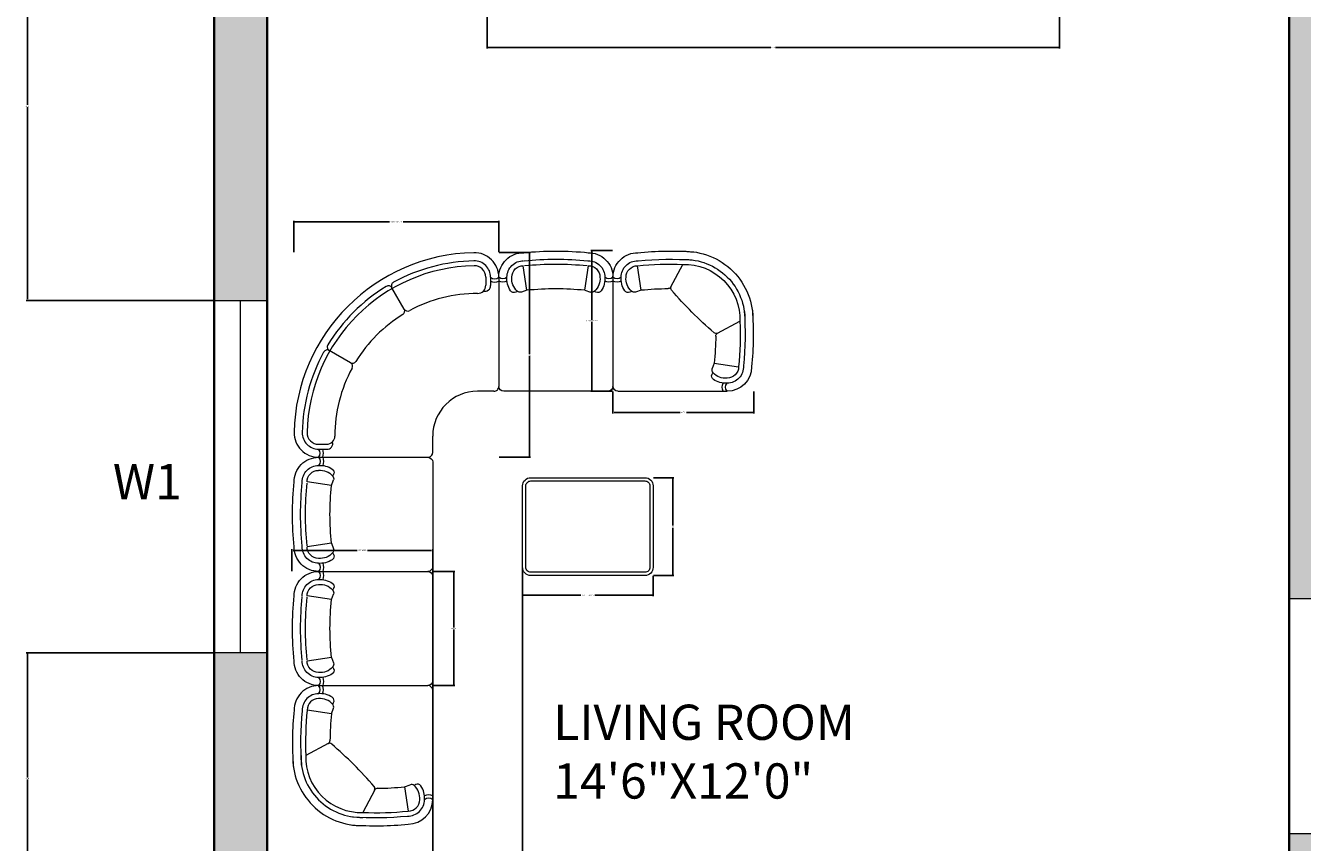
# Model space of a CAD drawing. Units: inches. Extents: x 5 to 421, y -617 to 43.
# Tile 6 of 15: x 5 to 223, y -385 to -246. Entities that reach past the tile are written whole.
import ezdxf

# ---------------------------------------------------------------- set-up
doc = ezdxf.new("R2010")
doc.units = ezdxf.units.IN
doc.header["$MEASUREMENT"] = 0
for name, color, linetype, lineweight in [('A-ANNO-DIMS', 2, 'Continuous', 18), ('A-ANNO-TEXT', 7, 'Continuous', 18), ('A-AREA-IDEN', 7, 'Continuous', 25), ('A-DOOR', 4, 'Continuous', 20), ('A-FURN', 8, 'Continuous', 13), ('A-GLAZ', 4, 'Continuous', 18), ('A-WALL', 7, 'Continuous', 35)]:
    doc.layers.add(name, color=color, linetype=linetype, lineweight=lineweight)
doc.layers.add('A-WALL-PATT', color=251, linetype='Continuous', lineweight=13, true_color=0x636466)
doc.styles.get("Standard").update_dxf_attribs({"font": 'arial.ttf'})
doc.dimstyles.get("Standard").update_dxf_attribs({"dimtxt": 0.18, "dimasz": 0.18, "dimexe": 0.18, "dimexo": 0.0625, "dimgap": 0.09, "dimtad": 0, "dimtih": 1, "dimtoh": 1, "dimdec": 0, "dimzin": 0, "dimdsep": 46, "dimlunit": 3, "dimtxsty": 'Standard', "dimcen": 0.09, "dimadec": 0, "dimazin": 0, "dimtfac": 1, "dimtdec": 0, "dimtofl": 0, "dimtmove": 0, "dimatfit": 3, "dimfxl": 1, "dimtolj": 1, "dimtzin": 0, "dimarcsym": 0})

# ---------------------------------------------------------------- blocks, each defined once
blk = doc.blocks.new('A$C707258B2')
at = {"color": 0}
for p, q in [((0.4042, 0.342), (1.0739, 0.342)), ((0.4042, 0.292), (0.4544, 0.292)), ((0.4042, 0.262), (0.4539, 0.262)), ((1.1039, 0.312), (1.1039, 0.212)), ((1.4789, -0.063), (1.3789, -0.063)), ((1.5089, -0.7628), (1.5089, -0.093)), ((0.5998, -0.2378), (0.4699, -0.3128)), ((0.9291, -0.5671), (0.8541, -0.697)), ((1.4289, -0.7628), (1.4289, -0.713)), ((1.4589, -0.7628), (1.4589, -0.7125))]:
    blk.add_line(p, q, dxfattribs=at)
for centre, radius, start, end in [((0.4042, 0.192), 0.15, 90, 181.17538), ((0.3779, 0.317), 0.0362, 316.39718, 43.60282), ((0.3679, 0.317), 0.0662, 337.82984, 22.17016), ((1.0739, 0.312), 0.03, 360, 90), ((0.4042, 0.192), 0.1, 90, 181.17538), ((0.4042, 0.192), 0.07, 90, 181.17538), ((0.4539, 0.212), 0.05, 360, 90), ((0.4548, 0.2564), 0.0357, 345.42616, 90.55549), ((1.3789, 0.212), 1.125, 181.17538, 268.82462), ((1.3789, 0.212), 1.075, 181.17538, 208.63569), ((1.3789, 0.212), 1.045, 181.17538, 268.82462), ((1.3789, 0.212), 0.875, 180, 208.40825), ((1.3789, 0.212), 0.275, 180, 270), ((1.4789, -0.093), 0.03, 360, 90), ((0.5873, -0.2162), 0.025, 300, 28.40825), ((0.6123, -0.2595), 0.025, 31.59175, 120), ((0.4574, -0.2912), 0.025, 208.63569, 300), ((0.4824, -0.3345), 0.025, 120, 211.36431), ((1.3789, 0.212), 0.875, 211.59175, 238.40825), ((1.3789, 0.212), 1.075, 211.36431, 238.63569), ((0.9075, -0.5546), 0.025, 330, 58.40825), ((0.9508, -0.5796), 0.025, 61.59175, 150), ((1.3789, 0.212), 0.875, 241.59175, 270), ((0.8324, -0.6845), 0.025, 238.63569, 330), ((0.8757, -0.7095), 0.025, 150, 241.36431), ((1.3789, -0.713), 0.05, 360, 90), ((1.4255, -0.7093), 0.0336, 354.63008, 109.38826), ((1.3789, 0.212), 1.075, 241.36431, 268.82462), ((1.3589, -0.7628), 0.15, 268.82462, 360), ((1.3589, -0.7628), 0.1, 268.82462, 360), ((1.3589, -0.7628), 0.07, 268.82462, 360), ((1.4839, -0.7988), 0.0662, 67.82984, 112.17016), ((1.4839, -0.789), 0.0362, 46.39718, 133.60282)]:
    blk.add_arc(centre, radius, start, end, dxfattribs=at)
blk = doc.blocks.new('A$C1352')
at = {"color": 0}
for points in [[(0.0027, 0.053), (0.0027, 0.553, -0.414214), (0.0527, 0.603), (0.7527, 0.603, -0.414214), (0.8027, 0.553), (0.8027, 0.053, -0.414214), (0.7527, 0.003), (0.0527, 0.003, -0.414214)], [(0.0227, 0.053), (0.0227, 0.553, -0.414214), (0.0527, 0.583), (0.7527, 0.583, -0.414214), (0.7827, 0.553), (0.7827, 0.053, -0.414214), (0.7527, 0.023), (0.0527, 0.023, -0.414214)]]:
    blk.add_lwpolyline(points, format="xyb", close=True, dxfattribs=at)
blk = doc.blocks.new('part 01')
at = {"color": 0}
for p, q in [((-669.8, 700), (0, 700)), ((30, 30), (30, 670)), ((-590.9, 527.1), (-739.8, 550)), ((-590.9, 527.1), (-578.5, 561.2)), ((-590.9, 172.9), (-739.8, 150)), ((-590.9, 172.9), (-578.5, 138.8)), ((-669.8, 0), (0, 0))]:
    blk.add_line(p, q, dxfattribs=at)
for centre, radius, start, end in [((-669.8, 550), 150, 90, 181.17538), ((-669.8, 550), 100, 90, 181.17538), ((-659.7, 517.8), 132.7, 56.08973, 95.61316), ((-696, 675), 36.2, 316.39718, 43.60282), ((-705.9, 675), 66.2, 337.82984, 22.17016), ((-599.7, 607.2), 25, 332.96082, 56.08973), ((0, 670), 30, 0, 90), ((1178.1, 350), 2007.9, 174.28354, 185.71646), ((-669.8, 550), 70, 90, 181.17538), ((-659.7, 517.8), 102.7, 42.00663, 95.61316), ((-624.8, 620), 53.2, 321.00172, 332.96082), ((-602, 569.8), 25, 340, 42.00663), ((1178.1, 350), 1957.9, 174.28354, 185.71646), ((1178.1, 350), 1927.9, 174.28354, 185.71646), ((1178.1, 350), 1777.9, 174.28354, 185.71646), ((-669.8, 150), 150, 178.82462, 270), ((-669.8, 150), 100, 178.82462, 270), ((-669.8, 150), 70, 178.82462, 270), ((-659.7, 182.2), 102.7, 264.38684, 317.99337), ((-599.7, 92.8), 25, 303.91027, 27.03918), ((-602, 130.2), 25, 317.99337, 20), ((-624.8, 80), 53.2, 27.03918, 38.99828), ((-659.7, 182.2), 132.7, 264.38684, 303.91027), ((-696, 25), 36.2, 316.39718, 43.60282), ((-705.9, 25), 66.2, 337.82984, 22.17016), ((0, 30), 30, 270, 0)]:
    blk.add_arc(centre, radius, start, end, dxfattribs=at)
blk = doc.blocks.new('part02')
at = {"color": 0}
for p, q in [((0, -669.8), (0, 0)), ((30, 30), (699.8, 30)), ((620.9, -142.9), (608.5, -108.8)), ((620.9, -142.9), (769.8, -120)), ((640.4, -325.6), (778.2, -398.9)), ((172.9, -590.9), (138.8, -578.5)), ((172.9, -590.9), (150, -739.8)), ((355.6, -610.4), (428.9, -748.2))]:
    blk.add_line(p, q, dxfattribs=at)
for centre, radius, start, end in [((30, 0), 30, 90, 180), ((726, 5), 56.2, 153.6122, 206.66656), ((726, 5), 36.2, 136.39718, 223.60282), ((699.8, -120), 150, 0, 90), ((629.7, -62.8), 25, 123.91027, 207.03918), ((654.8, -50), 53.2, 207.03918, 218.99828), ((689.7, -152.2), 102.7, 84.38684, 137.99337), ((689.3, -151.3), 131.7, 85.43775, 123.98866), ((699.5, -120.6), 100.6, 357.50055, 89.85796), ((699.8, -120), 70, 0, 90), ((632, -100.2), 25, 137.99337, 200), ((-1148.1, -320), 1777.9, 0.38365, 5.71646), ((-1228.2, -319.5), 2007.9, 357.73494, 5.70316), ((-1148.1, -320), 1957.9, 355.86566, 5.71646), ((-1148.1, -320), 2007.9, 355.81801, 5.71646), ((649.7, -308), 20, 180.38365, 242), ((2219.8, -2189.8), 2454.4, 130.6961, 139.3039), ((632.4, -344.1), 20, 62, 130.6961), ((439.4, -409.4), 418.9, 268.21809, 1.78191), ((439.4, -409.4), 368.9, 268.21809, 1.78191), ((439.4, -409.4), 338.9, 268.21809, 1.78191), ((182.2, -659.7), 132.7, 146.08973, 185.61316), ((92.8, -599.7), 25, 62.96082, 146.08973), ((182.2, -659.7), 102.7, 132.00663, 185.61316), ((80, -624.8), 53.2, 51.00172, 62.96082), ((130.2, -602), 25, 70, 132.00663), ((350, 1178.1), 1777.9, 264.28354, 269.61635), ((338, -619.7), 20, 28, 89.61635), ((374.1, -602.4), 20, 139.3039, 208), ((25, -696), 56.2, 63.33344, 116.3878), ((25, -696), 36.2, 46.39718, 133.60282), ((150, -669.8), 150, 180, 271.17538), ((150, -669.8), 100, 180, 271.17538), ((150, -669.8), 70, 180, 270), ((349.5, 1258.2), 2007.9, 264.29684, 272.26506), ((350, 1178.1), 1957.9, 264.28354, 274.13434), ((350, 1178.1), 2007.9, 264.28354, 274.18199)]:
    blk.add_arc(centre, radius, start, end, dxfattribs=at)
blk = doc.blocks.new('WINDOW-W1-60')
for p, q in [((0, 9), (60, 9)), ((0, 0), (0, 9)), ((60, 9), (60, 0)), ((0, 4.5), (60, 4.5)), ((60, 0), (0, 0))]:
    blk.add_line(p, q)
blk = doc.blocks.new('*D28')
at = {"layer": 'A-ANNO-DIMS', "color": 0, "lineweight": -2, "transparency": 16777216}
for p, q in [((50.66, -338.9), (50.66, -335.19)), ((50.84, -335.37), (61.75, -335.37)), ((74.44, -335.37), (63.53, -335.37)), ((74.62, -338.9), (74.62, -335.19))]:
    blk.add_line(p, q, dxfattribs=at)
at = {"layer": 'A-ANNO-DIMS', "color": 0, "transparency": 16777216}
for points in [[(50.84, -335.34), (50.84, -335.4), (50.66, -335.37)], [(74.44, -335.34), (74.44, -335.4), (74.62, -335.37)]]:
    blk.add_solid(points, dxfattribs=at)
at = {"layer": 'Defpoints', "color": 0, "transparency": 16777216}
for p in [(74.62, -335.37), (50.66, -338.96), (74.62, -338.96)]:
    blk.add_point(p, dxfattribs=at)
at = {"layer": 'A-ANNO-DIMS', "color": 0, "transparency": 16777216, "insert": (62.64, -335.37), "char_height": 0.18, "attachment_point": 5}
blk.add_mtext('\\A1;SEAT 24 TYP.', dxfattribs=at)
blk = doc.blocks.new('*D29')
at = {"layer": 'A-ANNO-DIMS', "color": 0, "lineweight": -2, "transparency": 16777216}
for p, q in [((74.69, -338.96), (78.4, -338.96)), ((78.22, -339.14), (78.22, -348.5)), ((78.22, -358.22), (78.22, -348.86)), ((74.69, -358.4), (78.4, -358.4))]:
    blk.add_line(p, q, dxfattribs=at)
at = {"layer": 'A-ANNO-DIMS', "color": 0, "transparency": 16777216}
for points in [[(78.19, -339.14), (78.25, -339.14), (78.22, -338.96)], [(78.19, -358.22), (78.25, -358.22), (78.22, -358.4)]]:
    blk.add_solid(points, dxfattribs=at)
at = {"layer": 'Defpoints', "color": 0, "transparency": 16777216}
for p in [(74.62, -338.96), (74.62, -358.4), (78.22, -358.4)]:
    blk.add_point(p, dxfattribs=at)
at = {"layer": 'A-ANNO-DIMS', "color": 0, "transparency": 16777216, "insert": (78.22, -348.68), "char_height": 0.18, "attachment_point": 5}
blk.add_mtext('\\A1;19 TYP.', dxfattribs=at)
blk = doc.blocks.new('*D30')
at = {"layer": 'A-ANNO-DIMS', "color": 0, "lineweight": -2, "transparency": 16777216}
for p, q in [((105.25, -284.32), (101.53, -284.32)), ((101.71, -284.5), (101.71, -296.11)), ((101.71, -308.1), (101.71, -296.48)), ((105.25, -308.28), (101.53, -308.28))]:
    blk.add_line(p, q, dxfattribs=at)
at = {"layer": 'A-ANNO-DIMS', "color": 0, "transparency": 16777216}
for points in [[(101.68, -284.5), (101.74, -284.5), (101.71, -284.32)], [(101.68, -308.1), (101.74, -308.1), (101.71, -308.28)]]:
    blk.add_solid(points, dxfattribs=at)
at = {"layer": 'Defpoints', "color": 0, "transparency": 16777216}
for p in [(105.31, -284.32), (101.71, -308.28), (105.31, -308.28)]:
    blk.add_point(p, dxfattribs=at)
at = {"layer": 'A-ANNO-DIMS', "color": 0, "transparency": 16777216, "insert": (101.71, -296.3), "char_height": 0.18, "attachment_point": 5}
blk.add_mtext('\\A1;END SEAT 24 TYP.', dxfattribs=at)
blk = doc.blocks.new('*D31')
at = {"layer": 'A-ANNO-DIMS', "color": 0, "lineweight": -2, "transparency": 16777216}
for p, q in [((105.31, -308.34), (105.31, -312.05)), ((129.27, -308.34), (129.27, -312.05)), ((105.49, -311.87), (116.76, -311.87)), ((129.09, -311.87), (117.82, -311.87))]:
    blk.add_line(p, q, dxfattribs=at)
at = {"layer": 'A-ANNO-DIMS', "color": 0, "transparency": 16777216}
for points in [[(105.49, -311.84), (105.49, -311.9), (105.31, -311.87)], [(129.09, -311.84), (129.09, -311.9), (129.27, -311.87)]]:
    blk.add_solid(points, dxfattribs=at)
at = {"layer": 'Defpoints', "color": 0, "transparency": 16777216}
for p in [(105.31, -308.28), (129.27, -308.28), (129.27, -311.87)]:
    blk.add_point(p, dxfattribs=at)
at = {"layer": 'A-ANNO-DIMS', "color": 0, "transparency": 16777216, "insert": (117.29, -311.87), "char_height": 0.18, "attachment_point": 5}
blk.add_mtext('\\A1;24 TYP.', dxfattribs=at)
blk = doc.blocks.new('*D32')
at = {"layer": 'A-ANNO-DIMS', "color": 0, "lineweight": -2, "transparency": 16777216}
for p, q in [((51, -284.59), (51, -279.25)), ((51.18, -279.43), (67.28, -279.43)), ((85.69, -279.43), (69.6, -279.43)), ((85.87, -284.59), (85.87, -279.25))]:
    blk.add_line(p, q, dxfattribs=at)
at = {"layer": 'A-ANNO-DIMS', "color": 0, "transparency": 16777216}
for points in [[(51.18, -279.4), (51.18, -279.46), (51, -279.43)], [(85.69, -279.4), (85.69, -279.46), (85.87, -279.43)]]:
    blk.add_solid(points, dxfattribs=at)
at = {"layer": 'Defpoints', "color": 0, "transparency": 16777216}
for p in [(85.87, -279.43), (51, -284.66), (85.87, -284.66)]:
    blk.add_point(p, dxfattribs=at)
at = {"layer": 'A-ANNO-DIMS', "color": 0, "transparency": 16777216, "insert": (68.44, -279.43), "char_height": 0.18, "attachment_point": 5}
blk.add_mtext('\\A1;CORNER SEAT 35', dxfattribs=at)
blk = doc.blocks.new('*D33')
at = {"layer": 'A-ANNO-DIMS', "color": 0, "lineweight": -2, "transparency": 16777216}
for p, q in [((85.93, -284.66), (91.28, -284.66)), ((91.1, -284.84), (91.1, -301.91)), ((91.1, -319.34), (91.1, -302.27)), ((85.93, -319.52), (91.28, -319.52))]:
    blk.add_line(p, q, dxfattribs=at)
at = {"layer": 'A-ANNO-DIMS', "color": 0, "transparency": 16777216}
for points in [[(91.07, -284.84), (91.13, -284.84), (91.1, -284.66)], [(91.07, -319.34), (91.13, -319.34), (91.1, -319.52)]]:
    blk.add_solid(points, dxfattribs=at)
at = {"layer": 'Defpoints', "color": 0, "transparency": 16777216}
for p in [(85.87, -284.66), (85.87, -319.52), (91.1, -319.52)]:
    blk.add_point(p, dxfattribs=at)
at = {"layer": 'A-ANNO-DIMS', "color": 0, "transparency": 16777216, "insert": (91.1, -302.09), "char_height": 0.18, "attachment_point": 5}
blk.add_mtext('\\A1;35', dxfattribs=at)
blk = doc.blocks.new('*D34')
at = {"layer": 'A-ANNO-DIMS', "color": 0, "lineweight": -2, "transparency": 16777216}
for p, q in [((89.92, -339.72), (89.92, -343.17)), ((112.14, -339.72), (112.14, -343.17)), ((90.1, -342.99), (99.84, -342.99)), ((111.96, -342.99), (102.23, -342.99))]:
    blk.add_line(p, q, dxfattribs=at)
at = {"layer": 'A-ANNO-DIMS', "color": 0, "transparency": 16777216}
for points in [[(90.1, -342.96), (90.1, -343.02), (89.92, -342.99)], [(111.96, -342.96), (111.96, -343.02), (112.14, -342.99)]]:
    blk.add_solid(points, dxfattribs=at)
at = {"layer": 'Defpoints', "color": 0, "transparency": 16777216}
for p in [(89.92, -339.66), (112.14, -339.66), (112.14, -342.99)]:
    blk.add_point(p, dxfattribs=at)
at = {"layer": 'A-ANNO-DIMS', "color": 0, "transparency": 16777216, "insert": (101.03, -342.99), "char_height": 0.18, "attachment_point": 5}
blk.add_mtext('\\A1;COFFEE TABLE 22', dxfattribs=at)
blk = doc.blocks.new('*D35')
at = {"layer": 'A-ANNO-DIMS', "color": 0, "lineweight": -2, "transparency": 16777216}
for p, q in [((112.2, -323), (115.65, -323)), ((115.47, -323.18), (115.47, -331.15)), ((115.47, -339.48), (115.47, -331.51)), ((112.2, -339.66), (115.65, -339.66))]:
    blk.add_line(p, q, dxfattribs=at)
at = {"layer": 'A-ANNO-DIMS', "color": 0, "transparency": 16777216}
for points in [[(115.44, -323.18), (115.5, -323.18), (115.47, -323)], [(115.44, -339.48), (115.5, -339.48), (115.47, -339.66)]]:
    blk.add_solid(points, dxfattribs=at)
at = {"layer": 'Defpoints', "color": 0, "transparency": 16777216}
for p in [(112.14, -323), (115.47, -323), (112.14, -339.66)]:
    blk.add_point(p, dxfattribs=at)
at = {"layer": 'A-ANNO-DIMS', "color": 0, "transparency": 16777216, "insert": (115.47, -331.33), "char_height": 0.18, "attachment_point": 5}
blk.add_mtext('\\A1;17', dxfattribs=at)
blk = doc.blocks.new('*D55')
at = {"layer": 'A-ANNO-DIMS', "color": 0, "lineweight": -2, "transparency": 16777216}
for p, q in [((370.48, 10.88), (420.4, 10.88)), ((420.22, 10.7), (420.22, -286.69)), ((420.22, -584.44), (420.22, -287.05)), ((169.48, -584.62), (420.4, -584.62))]:
    blk.add_line(p, q, dxfattribs=at)
at = {"layer": 'A-ANNO-DIMS', "color": 0, "transparency": 16777216}
for points in [[(420.19, 10.7), (420.25, 10.7), (420.22, 10.88)], [(420.19, -584.44), (420.25, -584.44), (420.22, -584.62)]]:
    blk.add_solid(points, dxfattribs=at)
at = {"layer": 'Defpoints', "color": 0, "transparency": 16777216}
for p in [(370.42, 10.88), (169.42, -584.62), (420.22, -584.62)]:
    blk.add_point(p, dxfattribs=at)
at = {"layer": 'A-ANNO-DIMS', "color": 0, "transparency": 16777216, "insert": (420.22, -286.87), "char_height": 0.18, "attachment_point": 5}
blk.add_mtext('\\A1;595.5', dxfattribs=at)
blk = doc.blocks.new('*D62')
at = {"layer": 'A-ANNO-DIMS', "color": 0, "lineweight": -2, "transparency": 16777216}
for p, q in [((37.36, -226.61), (5.44, -226.61)), ((5.62, -226.79), (5.62, -259.52)), ((5.62, -292.62), (5.62, -259.89)), ((37.36, -292.8), (5.44, -292.8))]:
    blk.add_line(p, q, dxfattribs=at)
at = {"layer": 'A-ANNO-DIMS', "color": 0, "transparency": 16777216}
for points in [[(5.59, -226.79), (5.65, -226.79), (5.62, -226.61)], [(5.59, -292.62), (5.65, -292.62), (5.62, -292.8)]]:
    blk.add_solid(points, dxfattribs=at)
at = {"layer": 'Defpoints', "color": 0, "transparency": 16777216}
for p in [(37.42, -226.61), (5.62, -292.8), (37.42, -292.8)]:
    blk.add_point(p, dxfattribs=at)
at = {"layer": 'A-ANNO-DIMS', "color": 0, "transparency": 16777216, "insert": (5.62, -259.71), "char_height": 0.18, "attachment_point": 5}
blk.add_mtext('\\A1;66.19', dxfattribs=at)
blk = doc.blocks.new('*D63')
at = {"layer": 'A-ANNO-DIMS', "color": 0, "lineweight": -2, "transparency": 16777216}
for p, q in [((37.36, -352.8), (5.44, -352.8)), ((5.62, -352.98), (5.62, -374.03)), ((5.62, -395.44), (5.62, -374.39)), ((37.36, -395.62), (5.44, -395.62))]:
    blk.add_line(p, q, dxfattribs=at)
at = {"layer": 'A-ANNO-DIMS', "color": 0, "transparency": 16777216}
for points in [[(5.59, -352.98), (5.65, -352.98), (5.62, -352.8)], [(5.59, -395.44), (5.65, -395.44), (5.62, -395.62)]]:
    blk.add_solid(points, dxfattribs=at)
at = {"layer": 'Defpoints', "color": 0, "transparency": 16777216}
for p in [(37.42, -352.8), (5.62, -395.62), (37.42, -395.62)]:
    blk.add_point(p, dxfattribs=at)
at = {"layer": 'A-ANNO-DIMS', "color": 0, "transparency": 16777216, "insert": (5.62, -374.21), "char_height": 0.18, "attachment_point": 5}
blk.add_mtext('\\A1;42.82', dxfattribs=at)
blk = doc.blocks.new('*D76')
at = {"layer": 'A-ANNO-DIMS', "color": 0, "lineweight": -2, "transparency": 16777216}
for p, q in [((83.88, -217.98), (83.88, -249.9)), ((181.3, -217.98), (181.3, -249.9)), ((84.06, -249.72), (132.19, -249.72)), ((181.12, -249.72), (132.98, -249.72))]:
    blk.add_line(p, q, dxfattribs=at)
at = {"layer": 'A-ANNO-DIMS', "color": 0, "transparency": 16777216}
for points in [[(84.06, -249.69), (84.06, -249.75), (83.88, -249.72)], [(181.12, -249.69), (181.12, -249.75), (181.3, -249.72)]]:
    blk.add_solid(points, dxfattribs=at)
at = {"layer": 'Defpoints', "color": 0, "transparency": 16777216}
for p in [(83.88, -217.92), (181.3, -217.92), (83.88, -249.72)]:
    blk.add_point(p, dxfattribs=at)
at = {"layer": 'A-ANNO-DIMS', "color": 0, "transparency": 16777216, "insert": (132.59, -249.72), "char_height": 0.18, "attachment_point": 5}
blk.add_mtext('\\A1;97.42', dxfattribs=at)
blk = doc.blocks.new('*D78')
at = {"layer": 'A-ANNO-DIMS', "color": 0, "lineweight": -2, "transparency": 16777216}
for p, q in [((74.62, -338.19), (74.62, -616.6)), ((89.92, -338.33), (89.92, -616.6)), ((74.8, -616.42), (81.96, -616.42)), ((89.74, -616.42), (82.59, -616.42))]:
    blk.add_line(p, q, dxfattribs=at)
at = {"layer": 'A-ANNO-DIMS', "color": 0, "transparency": 16777216}
for points in [[(74.8, -616.39), (74.8, -616.45), (74.62, -616.42)], [(89.74, -616.39), (89.74, -616.45), (89.92, -616.42)]]:
    blk.add_solid(points, dxfattribs=at)
at = {"layer": 'Defpoints', "color": 0, "transparency": 16777216}
for p in [(74.62, -338.13), (89.92, -338.27), (89.92, -616.42)]:
    blk.add_point(p, dxfattribs=at)
at = {"layer": 'A-ANNO-DIMS', "color": 0, "transparency": 16777216, "insert": (82.27, -616.42), "char_height": 0.18, "attachment_point": 5}
blk.add_mtext('\\A1;15.3', dxfattribs=at)

msp = doc.modelspace()

# ---------------------------------------------------------------- hatches: boundary and pattern name
at = {"layer": 'A-WALL-PATT'}
h = msp.add_hatch(color=256, dxfattribs=at)
h.dxf.hatch_style = 1
h.paths.add_polyline_path([(46.4196, -88.1188), (37.4196, -88.1188), (37.4196, -166.6119), (46.4196, -166.6119), (46.4196, -122.6188), (135.4196, -122.6188), (135.4196, -120.3688), (135.4196, -118.1188), (46.4196, -118.1188)])
h.paths.add_polyline_path([(82.4196, 10.8812), (37.4196, 10.8812), (37.4196, -28.1188), (46.4196, -28.1188), (46.4196, 1.8812), (82.4196, 1.8812)])
h.paths.add_polyline_path([(215.5968, 10.8812), (142.4196, 10.8812), (142.4196, 1.8812), (178.4196, 1.8812), (178.4196, -118.1188), (175.4196, -118.1188), (175.4196, -122.6188), (182.9196, -122.6188), (182.9196, -80.6188), (211.9196, -80.6188), (211.9196, -78.3688), (211.9196, -76.1188), (182.9196, -76.1188), (182.9196, 1.8812), (215.5968, 1.8812)])
h.paths.add_polyline_path([(274.4196, 10.8812), (239.5968, 10.8812), (239.5968, 1.8812), (242.9196, 1.8812), (242.9196, -76.1188), (239.9196, -76.1188), (239.9196, -80.6188), (242.9196, -80.6188), (242.9196, -83.6188), (247.4196, -83.6188), (247.4196, 1.8812), (274.4196, 1.8812)])
h.paths.add_polyline_path([(370.4196, 10.8812), (334.4196, 10.8812), (334.4196, 1.8812), (361.4196, 1.8812), (361.4196, -28.1188), (370.4196, -28.1188)])
h.paths.add_polyline_path([(370.4196, -88.1188), (361.4196, -88.1188), (361.4196, -118.1188), (247.4196, -118.1188), (247.4196, -115.1188), (242.9196, -115.1188), (242.9196, -118.1188), (220.4196, -118.1188), (220.4196, -158.6188), (224.9196, -158.6188), (224.9196, -122.6188), (326.9196, -122.6188), (326.9196, -170.7662), (331.4196, -170.7662), (331.4196, -122.6188), (370.4196, -122.6188)])
h.paths.add_polyline_path([(388.4196, -122.6188), (388.4196, -118.1188), (379.4196, -118.1188), (379.4196, -122.6188), (379.4196, -154.8688), (388.4196, -154.8688)])
h.paths.add_polyline_path([(388.4196, -214.8688), (379.4196, -214.8688), (379.4196, -247.1188), (388.4196, -247.1188)])
h.paths.add_polyline_path([(371.0265, -242.6188), (331.4196, -242.6188), (331.4196, -239.6188), (326.9196, -239.6188), (326.9196, -242.6188), (224.9196, -242.6188), (224.9196, -206.6188), (220.4196, -206.6188), (220.4196, -343.6188), (224.9196, -343.6188), (229.4196, -343.6188), (229.4196, -247.1188), (261.5265, -247.1188), (261.5265, -276.1188), (263.7765, -276.1188), (266.0265, -276.1188), (266.0265, -247.1188), (362.0265, -247.1188), (362.0265, -265.1188), (371.0265, -265.1188), (371.0265, -247.1188)])
h.paths.add_polyline_path([(371.0265, -289.1188), (362.0265, -289.1188), (362.0265, -307.1188), (266.0265, -307.1188), (266.0265, -304.1188), (261.5265, -304.1188), (261.5265, -307.1188), (261.5265, -311.6188), (362.0265, -311.6188), (362.0265, -353.6188), (371.0265, -353.6188)])
h.paths.add_polyline_path([(371.0265, -413.6188), (362.0265, -413.6188), (362.0265, -455.6188), (325.7231, -455.6188), (325.7231, -464.6188), (361.4196, -464.6188), (371.0265, -464.6188)])
h.paths.add_polyline_path([(265.7231, -455.6188), (229.4196, -455.6188), (229.4196, -383.6188), (220.4196, -383.6188), (220.4196, -386.6188), (207.4649, -386.6188), (207.4649, -395.6188), (220.4196, -395.6188), (220.4196, -455.6188), (216.0568, -455.6188), (216.0568, -464.6188), (265.7231, -464.6188)])
h.paths.add_polyline_path([(169.4196, -386.6188), (137.9196, -386.6188), (137.9196, -395.6188), (160.4196, -395.6188), (160.4196, -424.2032), (169.4196, -424.2032)])
h.paths.add_polyline_path([(169.4196, -453.7423), (160.4196, -453.7423), (160.4196, -464.6188), (169.4196, -464.6188)])
h.paths.add_polyline_path([(46.4196, -575.6188), (37.4196, -575.6188), (37.4196, -584.6188), (46.4196, -584.6188)])
h.paths.add_polyline_path([(169.4196, -575.6188), (160.4196, -575.6188), (160.4196, -579.5504), (160.4196, -584.6188), (169.4196, -584.6188)])
h.paths.add_polyline_path([(46.4196, -226.6119), (37.4196, -226.6119), (37.4196, -292.8008), (46.4196, -292.8008)])
h.paths.add_polyline_path([(46.4196, -352.8008), (37.4196, -352.8008), (37.4196, -395.6188), (77.9196, -395.6188), (77.9196, -386.6188), (46.4196, -386.6188)])

# ---------------------------------------------------------------- linework, layer by layer
at = {"layer": 'A-DOOR'}
for p, q in [((224.9196, -343.6188), (220.4196, -343.6188)), ((220.4196, -383.6188), (229.4196, -383.6188))]:
    msp.add_line(p, q, dxfattribs=at)
at = {"layer": 'A-WALL'}
for p, q in [((37.4196, 10.8812), (37.4196, -584.6188)), ((46.4196, -122.6188), (46.4196, -386.6188)), ((220.4196, -206.6188), (220.4196, -386.6188))]:
    msp.add_line(p, q, dxfattribs=at)

# ---------------------------------------------------------------- block references
at = {"layer": 'A-FURN', "ltscale": 0.03}
for name, p, xscale, yscale, zscale, rotation in [('A$C707258B2', (76.3725, -277.6211), 27.76864329666651, 27.76864329666651, 27.76864329666651, 270.0000000000033), ('part 01', (105.308, -307.4431), -0.0277686432966665, 0.0277686432966665, 0.0277686432966665, 90), ('part02', (105.308, -307.4431), -0.0277686432966665, 0.0277686432966665, 0.0277686432966665, 180), ('part 01', (73.7906, -319.5225), -0.0277686432966665, 0.0277686432966665, 0.0277686432966665, 180), ('part 01', (73.7906, -338.9606), -0.0277686432966665, 0.0277686432966665, 0.0277686432966665, 180), ('part02', (73.7906, -358.3986), 0.0277686432966665, 0.0277686432966665, 0.0277686432966665, 270.0000000000033)]:
    msp.add_blockref(name, p, dxfattribs=dict(at, xscale=xscale, yscale=yscale, zscale=zscale, rotation=rotation))
at = {"layer": 'A-FURN', "ltscale": 0.03, "xscale": 27.76864329666651, "yscale": 27.76864329666651, "zscale": 27.76864329666651}
msp.add_blockref('A$C1352', (89.8492, -339.7402), dxfattribs=at)
at = {"layer": 'A-GLAZ', "rotation": 90.00000000000003}
msp.add_blockref('WINDOW-W1-60', (46.4196, -352.8008), dxfattribs=at)

# ---------------------------------------------------------------- texts
at = {"layer": 'A-ANNO-TEXT', "insert": (20.1784, -320.6585), "char_height": 6, "attachment_point": 1}
msp.add_mtext('W1', dxfattribs=at)
at = {"layer": 'A-AREA-IDEN', "insert": (95.14, -361.6444), "char_height": 6, "attachment_point": 1}
msp.add_mtext('LIVING ROOM\\P14\'6"X12\'0"', dxfattribs=at)

# ---------------------------------------------------------------- dimensions: what is measured, and where the dimension line sits
at = {"layer": 'A-ANNO-DIMS'}
for base, p1, p2, angle, override, picture, middle in [((420.2196, -584.6188), (370.4196, 10.8812), (169.4196, -584.6188), 90, {"dimdec": 1, "dimlfac": 1, "dimrnd": 0, "dimzin": 0, "dimdsep": 46, "dimlunit": 2}, '*D55', (420.2196, -286.8688)), ((83.8765, -249.7206), (181.2958, -217.9206), (83.8765, -217.9206), 180, {"dimdec": 2, "dimlfac": 1, "dimrnd": 0, "dimzin": 0, "dimdsep": 46, "dimlunit": 2}, '*D76', (132.5862, -249.7206)), ((5.6196, -292.8008), (37.4196, -226.6119), (37.4196, -292.8008), 90, {"dimdec": 2, "dimlfac": 1, "dimrnd": 0, "dimzin": 0, "dimdsep": 46, "dimlunit": 2}, '*D62', (5.6196, -259.7064)), ((91.0999, -319.5225), (85.87, -284.6565), (85.87, -319.5225), 270, {"dimdec": 0, "dimlfac": 1, "dimrnd": 0, "dimzin": 0, "dimdsep": 46, "dimlunit": 2}, '*D33', (91.0999, -302.0895)), ((115.471, -322.9959), (112.1387, -339.6571), (112.1387, -322.9959), 90, {"dimdec": 0, "dimlfac": 1, "dimrnd": 0, "dimzin": 0, "dimdsep": 46, "dimlunit": 2}, '*D35', (115.471, -331.3265)), ((5.6196, -395.6188), (37.4196, -352.8008), (37.4196, -395.6188), 90, {"dimdec": 2, "dimlfac": 1, "dimrnd": 0, "dimzin": 0, "dimdsep": 46, "dimlunit": 2}, '*D63', (5.6196, -374.2098))]:
    dim = msp.add_linear_dim(base=base, p1=p1, p2=p2, angle=angle, dimstyle='Standard', override=override, dxfattribs=at)
    dim.commit()
    dim.dimension.update_dxf_attribs({"geometry": picture, "text_midpoint": middle})
for base, p1, p2, angle, text, picture, middle in [((85.87, -279.4266), (51.0039, -284.6565), (85.87, -284.6565), 0, 'CORNER SEAT <>', '*D32', (68.437, -279.4266)), ((101.7139, -308.2762), (105.308, -284.3154), (105.308, -308.2762), 270, 'END SEAT <> TYP.', '*D30', (101.7139, -296.2958)), ((78.2188, -358.3986), (74.6237, -338.9606), (74.6237, -358.3986), 270, '<> TYP.', '*D29', (78.2188, -348.6796))]:
    dim = msp.add_linear_dim(base=base, p1=p1, p2=p2, angle=angle, text=text, dimstyle='Standard', override={"dimdec": 0, "dimlfac": 1, "dimrnd": 0, "dimzin": 0, "dimdsep": 46, "dimlunit": 2}, dxfattribs=at)
    dim.commit()
    dim.dimension.update_dxf_attribs({"geometry": picture, "text_midpoint": middle})
for base, p1, p2, text, picture, middle in [((129.2688, -311.8703), (105.308, -308.2762), (129.2688, -308.2762), '<> TYP.', '*D31', (117.2884, -311.8703)), ((74.6237, -335.3654), (50.6563, -338.9606), (74.6237, -338.9606), 'SEAT <> TYP.', '*D28', (62.64, -335.3654)), ((112.1387, -342.9893), (89.9238, -339.6571), (112.1387, -339.6571), 'COFFEE TABLE <>', '*D34', (101.0313, -342.9893))]:
    dim = msp.add_linear_dim(base=base, p1=p1, p2=p2, text=text, dimstyle='Standard', override={"dimdec": 0, "dimlfac": 1, "dimrnd": 0, "dimzin": 0, "dimdsep": 46, "dimlunit": 2}, dxfattribs=at)
    dim.commit()
    dim.dimension.update_dxf_attribs({"geometry": picture, "text_midpoint": middle})
dim = msp.add_linear_dim(base=(89.9238, -616.4188), p1=(74.6237, -338.1275), p2=(89.9238, -338.2687), dimstyle='Standard', override={"dimdec": 1, "dimlfac": 1, "dimrnd": 0, "dimzin": 0, "dimdsep": 46, "dimlunit": 2}, dxfattribs=at)
dim.commit()
dim.dimension.update_dxf_attribs({"geometry": '*D78', "text_midpoint": (82.2737, -616.4188)})

doc.saveas('drawing.dxf')
